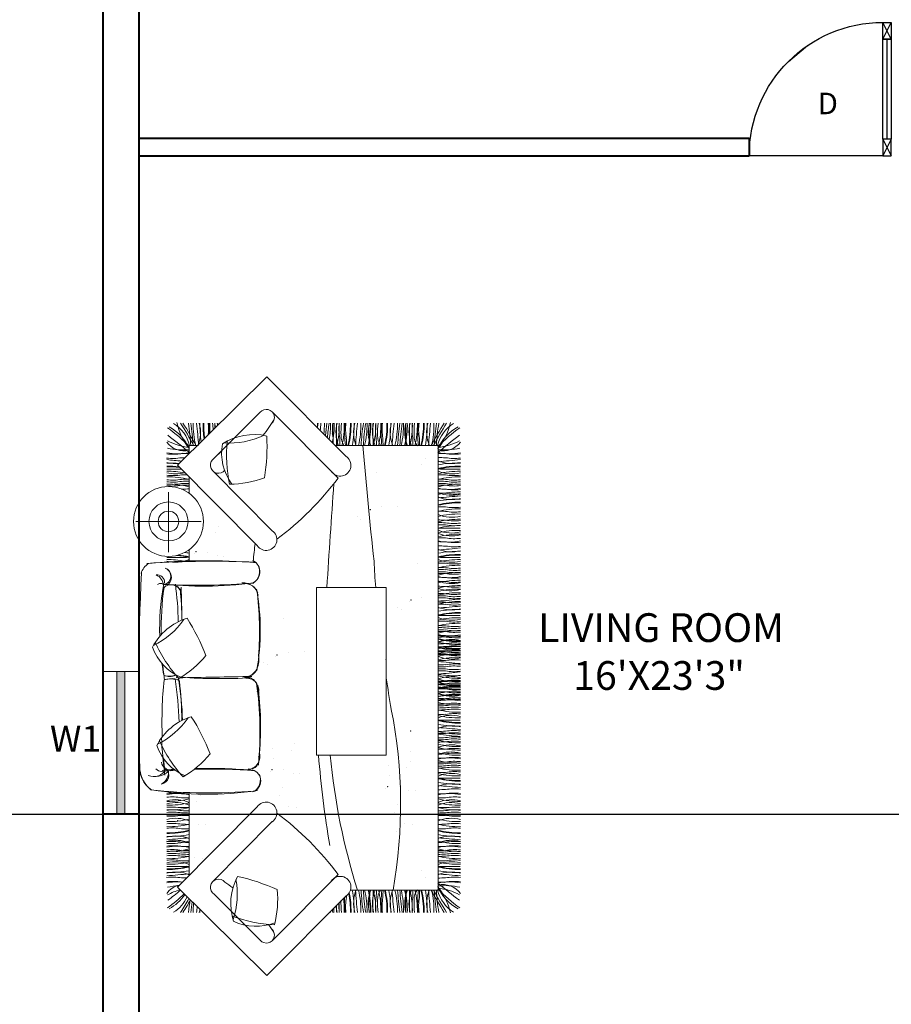
# Model space of a CAD drawing. Units: inches. Extents: x 182 to 1022, y -617 to 111.
# Tile 28 of 33: x 615 to 836, y -337 to -87. Entities that reach past the tile are written whole.
import ezdxf

# ---------------------------------------------------------------- set-up
doc = ezdxf.new("R2010")
doc.units = ezdxf.units.IN
doc.header["$MEASUREMENT"] = 0
for name, color, linetype, lineweight in [('A-ANNO-DIMS', 2, 'Continuous', 18), ('A-ANNO-IDEN', 1, 'Continuous', 18), ('A-AREA-IDEN', 8, 'Continuous', 18), ('A-GLAZ-PATT', 5, 'Continuous', 13), ('door', 2, 'Continuous', 25), ('wall', 1, 'Continuous', 40), ('wind', 5, 'Continuous', 20)]:
    doc.layers.add(name, color=color, linetype=linetype, lineweight=lineweight)
doc.layers.add('furniture', color=50, linetype='Continuous', lineweight=15, transparency=0.8)
doc.styles.get("Standard").update_dxf_attribs({"font": 'arial.ttf'})
doc.dimstyles.get("Standard").update_dxf_attribs({"dimtxt": 0.18, "dimasz": 0.18, "dimexe": 0.18, "dimexo": 0.0625, "dimgap": 0.09, "dimtad": 0, "dimtih": 1, "dimtoh": 1, "dimdec": 1, "dimzin": 0, "dimdsep": 46, "dimlunit": 4, "dimtxsty": 'Standard', "dimcen": 0.09, "dimadec": 0, "dimazin": 0, "dimtfac": 1, "dimtdec": 1, "dimtofl": 0, "dimtmove": 0, "dimatfit": 3, "dimfxl": 1, "dimtolj": 1, "dimtzin": 0, "dimarcsym": 0})

# ---------------------------------------------------------------- blocks, each defined once
blk = doc.blocks.new('A$C2D7661C6')
for p, q in [((0, 700), (50, 800)), ((50, 700), (0, 800)), ((25, 700), (25, 100)), ((50, 100), (0, 0)), ((0, 100), (50, 0))]:
    blk.add_line(p, q)
for points in [[(0, 700), (50, 700), (50, 800), (0, 800)], [(0, 100), (50, 100), (50, 700), (0, 700)], [(0, 100), (50, 100), (50, 0), (0, 0)]]:
    blk.add_lwpolyline(points, close=True)
blk.add_arc((50, 0), 800, 0, 90)
blk = doc.blocks.new('A$C7F556C88')
for p, q in [((615.7, 565.7), (500.3, 661.3)), ((50, 0), (850, 0))]:
    blk.add_line(p, q)
blk.add_blockref('A$C2D7661C6', (0, 0))
blk = doc.blocks.new('LOUNGE-SEATING-GROUP')
for p, q in [((114.94, 73.89), (114.94, 82.17)), ((114.94, 73.89), (107.2, 73.89)), ((114.94, 73.89), (114.94, 65.61)), ((114.94, 73.89), (122.39, 73.89)), ((22.37, 71.64), (0, 48.98)), ((22.37, 71.64), (42.71, 51.42)), ((23.45, 70.43), (23.45, 70.43)), ((23.45, 70.43), (23.45, 70.43)), ((23.45, 70.43), (23.45, 70.43)), ((24.81, 70.1), (24.81, 70.1)), ((24.81, 70.1), (24.81, 70.1)), ((24.81, 70.1), (24.81, 70.1)), ((38.82, 71.99), (38.82, 71.99)), ((41.95, 71.18), (41.95, 71.18)), ((44.62, 71.4), (44.62, 71.4)), ((129.17, 71.64), (108.83, 51.42)), ((129.17, 71.64), (151.54, 48.98)), ((131, 70.1), (131, 70.1)), ((131, 70.1), (131, 70.1)), ((131, 70.1), (131, 70.1)), ((132.36, 70.43), (132.36, 70.43)), ((132.36, 70.43), (132.36, 70.43)), ((132.36, 70.43), (132.36, 70.43)), ((25.37, 68.66), (46.02, 68.66)), ((27.79, 69.24), (27.79, 69.24)), ((27.79, 69.24), (27.79, 69.24)), ((29.83, 67.31), (29.83, 67.31)), ((32.6, 69.72), (32.6, 69.72)), ((34.6, 69.02), (34.6, 69.02)), ((39.15, 68.69), (39.15, 68.69)), ((104.96, 68.66), (107.81, 68.66)), ((106.87, 67.34), (106.87, 67.34)), ((122.07, 68.66), (126.17, 68.66)), ((132.11, 68.66), (134.14, 68.66)), ((134.14, 68.66), (134.14, 66.6)), ((29.68, 65.32), (29.68, 65.32)), ((38.28, 66.24), (38.28, 66.24)), ((44, 66.69), (44, 66.69)), ((45.68, 65.87), (45.68, 65.87)), ((23.81, 62.71), (38.96, 47.66)), ((38.14, 64.53), (38.14, 64.53)), ((107.19, 64.04), (107.19, 64.04)), ((127.73, 62.71), (112.58, 47.66)), ((20.57, 62.3), (8.95, 50.67)), ((20.57, 62.3), (16.28, 58)), ((106.19, 59.88), (106.19, 59.88)), ((106.32, 61.59), (106.32, 61.59)), ((112.04, 62.04), (112.04, 62.04)), ((113.72, 61.22), (113.72, 61.22)), ((130.97, 62.3), (142.59, 50.67)), ((130.97, 62.3), (132.83, 60.43)), ((136.11, 57.16), (142.59, 50.67)), ((12.73, 54.45), (8.95, 50.67)), ((0, 48.98), (20.08, 29.02)), ((25.6, 30.99), (8.82, 47.69)), ((51.77, 48.08), (51.77, 48.08)), ((57.56, 47.49), (57.56, 47.49)), ((78.69, 48.81), (78.69, 48.81)), ((78.69, 48.81), (78.69, 48.81)), ((79.3, 49.74), (79.3, 49.74)), ((79.3, 49.74), (79.3, 49.74)), ((125.94, 30.99), (142.72, 47.69)), ((151.54, 48.98), (131.46, 29.02)), ((40.73, 45.33), (40.73, 45.33)), ((40.73, 45.33), (40.73, 45.33)), ((45.54, 45.81), (45.54, 45.81)), ((47.55, 45.11), (47.55, 45.11)), ((54.89, 47.26), (54.89, 47.26)), ((80.67, 46.7), (80.67, 46.7)), ((42.77, 43.4), (42.77, 43.4)), ((52.09, 44.78), (52.09, 44.78)), ((56.94, 42.77), (56.94, 42.77)), ((81.89, 43.62), (81.89, 43.62)), ((90.41, 44.74), (90.41, 44.74)), ((42.63, 41.41), (42.63, 41.41)), ((51.09, 40.62), (51.09, 40.62)), ((51.22, 42.33), (51.22, 42.33)), ((58.62, 41.96), (58.62, 41.96)), ((81.95, 39.42), (81.95, 39.42)), ((55.77, 18.79), (55.77, 36.47)), ((55.77, 36.47), (98.22, 36.47)), ((98.22, 36.47), (98.22, 18.79)), ((137.17, 32.68), (137.17, 32.68)), ((137.71, 32.64), (137.71, 32.64)), ((134.14, 31.68), (134.14, 5.69)), ((21.66, 5.69), (21.66, 27.82)), ((115.51, 25.24), (115.51, 25.24)), ((115.51, 25.24), (115.51, 25.24)), ((116.12, 26.16), (116.12, 26.16)), ((116.12, 26.16), (116.12, 26.16)), ((18.1, 23.39), (18.1, 23.39)), ((18.64, 23.43), (18.64, 23.43)), ((117.49, 23.12), (117.49, 23.12)), ((137.17, 23.43), (137.17, 23.43)), ((137.71, 23.39), (137.71, 23.39)), ((118.71, 20.04), (118.71, 20.04)), ((127.23, 21.16), (127.23, 21.16)), ((47.45, 18.85), (47.45, 18.85)), ((50.58, 18.04), (50.58, 18.04)), ((53.25, 18.27), (53.25, 18.27)), ((98.22, 18.79), (55.77, 18.79)), ((36.42, 16.11), (36.42, 16.11)), ((36.42, 16.11), (36.42, 16.11)), ((41.23, 16.58), (41.23, 16.58)), ((43.23, 15.88), (43.23, 15.88)), ((47.78, 15.55), (47.78, 15.55)), ((93.22, 15.87), (93.22, 15.87)), ((93.22, 15.87), (93.22, 15.87)), ((118.77, 15.84), (118.77, 15.84)), ((18.1, 14.15), (18.1, 14.15)), ((18.64, 14.19), (18.64, 14.19)), ((38.46, 14.18), (38.46, 14.18)), ((46.91, 13.1), (46.91, 13.1)), ((52.63, 13.55), (52.63, 13.55)), ((54.31, 12.74), (54.31, 12.74)), ((56.63, 12.7), (56.63, 12.7)), ((92.6, 14.94), (92.6, 14.94)), ((92.6, 14.94), (92.6, 14.94)), ((94.58, 12.83), (94.58, 12.83)), ((137.17, 14.19), (137.17, 14.19)), ((137.71, 14.15), (137.71, 14.15)), ((38.31, 12.19), (38.31, 12.19)), ((46.77, 11.39), (46.77, 11.39)), ((104.33, 10.87), (104.33, 10.87)), ((24.84, 8.76), (24.84, 8.76)), ((26.54, 9.97), (26.54, 9.97)), ((95.8, 9.74), (95.8, 9.74)), ((129.27, 9.97), (129.27, 9.97)), ((130.96, 8.76), (130.96, 8.76)), ((134.14, 5.69), (21.66, 5.69)), ((39.44, 5.69), (134.14, 5.69)), ((95.87, 5.55), (95.87, 5.55)), ((23.45, 3.92), (23.45, 3.92)), ((23.45, 3.92), (23.45, 3.92)), ((23.45, 3.92), (23.45, 3.92)), ((24.81, 4.25), (24.81, 4.25)), ((24.81, 4.25), (24.81, 4.25)), ((24.81, 4.25), (24.81, 4.25)), ((69.92, 3.92), (69.92, 3.92)), ((70.05, 3.92), (70.05, 3.92)), ((73.89, 3.92), (73.89, 3.92)), ((81.92, 3.92), (81.92, 3.92)), ((85.76, 3.92), (85.76, 3.92)), ((85.89, 3.92), (85.89, 3.92)), ((131, 4.25), (131, 4.25)), ((131, 4.25), (131, 4.25)), ((131, 4.25), (131, 4.25)), ((132.36, 3.92), (132.36, 3.92)), ((132.36, 3.92), (132.36, 3.92)), ((132.36, 3.92), (132.36, 3.92))]:
    blk.add_line(p, q)
for radius in [8.84, 4.94, 2.61]:
    blk.add_circle((114.94, 73.89), radius)
for centre, radius, start, end in [((52.76, 74.33), 6.91, 83.8792, 147.1093), ((53.34, 72.78), 8.45, 98.6549, 138.7104), ((71.79, -550.87), 632.32, 87.2697, 91.7875), ((100.54, 76.54), 4.47, 31.8817, 73.9672), ((133.78, 64.16), 87.87, 170.8079, 188.3514), ((189.05, 63.59), 142.82, 174.0627, 184.6253), ((53.65, 77.61), 3.29, 154.8715, 246.7247), ((55.6, 77.33), 5.2, 161.2473, 221.1348), ((87.47, 65.64), 13.03, 109.4501, 156.7699), ((76.48, 64.92), 14.61, 17.0126, 62.9429), ((101.32, 86.34), 19.77, 205.9005, 235.6513), ((-54.46, 64.25), 159.48, 355.4325, 5.431), ((-129.18, 62.85), 234.07, 357.3143, 3.933), ((51.47, 77.28), 3.39, 207.8433, 279.8684), ((50.67, 76.05), 2.22, 189.2916, 317.6289), ((73.49, 44.66), 34.51, 114.0815, 132.2768), ((62.54, 64.57), 13.03, 109.4501, 156.7699), ((63.55, -12.93), 88.65, 92.2017, 98.3067), ((54.24, 75.33), 2.63, 137.7203, 204.4461), ((64.36, -31.32), 106.86, 95.0871, 96.7491), ((-77.45, 64.06), 129.9, 3.7101, 5.0653), ((54.5, 73.24), 2.5, 100.6216, 199.193), ((51.55, 63.85), 14.61, 17.0126, 62.9429), ((76.39, 85.27), 19.77, 205.9005, 235.6513), ((64.36, -31.32), 106.86, 84.3639, 92.1219), ((67.78, 73.23), 7.3, 344.0479, 14.2061), ((69.17, 73.11), 6, 351.5362, 18.3493), ((87.05, -6.17), 81.95, 95.7795, 98.522), ((98.42, 45.73), 34.51, 114.0815, 132.2768), ((78.62, 73.56), 2.96, 149.8319, 209.468), ((80.09, 73.77), 4.35, 163.3108, 202.6164), ((87.64, 12.43), 63.7, 97.803, 100.4557), ((87.64, 12.43), 63.7, 79.9466, 91.5903), ((87.05, -6.17), 81.95, 82.1551, 90.5585), ((96.33, 73.24), 2.6, 276.1174, 43.1189), ((189.77, 65.05), 91.22, 172.9836, 187.989), ((98.67, 78.16), 2.97, 271.184, 337.8216), ((97.61, 75.78), 1.68, 314.3938, 33.5856), ((303.26, 66.39), 204.45, 177.5073, 183.9592), ((101.1, 75.54), 2.22, 194.7814, 337.5922), ((99.47, 76.82), 1.96, 268.0108, 6.5585), ((23.91, 77.56), 9.3, 212.2712, 244.6274), ((26.62, 78.75), 10.9, 207.3033, 235.7016), ((48.18, 96.13), 38.02, 215.3153, 223.6457), ((157.47, 180.45), 174.58, 217.5441, 218.8901), ((9.21, 67.69), 12.92, 14.6792, 29.865), ((17.54, 69.88), 5.5, 12.9777, 54.0943), ((7.21, 70.59), 15.55, 2.5322, 13.2785), ((9.4, 71.55), 14.33, 355.1756, 11.2455), ((11.06, 72.81), 12.79, 349.9349, 6.8829), ((12.13, 72.82), 12.79, 349.9349, 6.8829), ((-225.09, 48.88), 251.6, 4.5146, 5.8017), ((17.36, 72.06), 8.84, 337.3098, 14.8613), ((54.69, 73.85), 28.62, 179.0195, 190.4039), ((48.4, 73.82), 21.55, 178.6331, 193.8573), ((48.56, 73.82), 21.55, 178.6331, 193.8573), ((-156.89, 73.02), 184.52, 358.628, 0.3934), ((19.99, 72.06), 8.84, 337.3098, 14.8613), ((49.71, 73.82), 21.55, 178.6331, 193.8573), ((16.48, 72.8), 12.79, 349.9349, 6.8829), ((51.14, 73.82), 21.55, 178.6331, 193.8573), ((17.61, 72.81), 12.79, 349.9349, 6.8829), ((18.12, 72.81), 12.79, 349.9349, 6.8829), ((18.68, 72.81), 12.79, 349.9349, 6.8829), ((52.99, 73.83), 21.55, 178.6331, 193.8573), ((19.1, 72.81), 12.79, 349.9349, 6.8829), ((18.41, 71.55), 14.33, 348.4112, 11.2455), ((20.08, 72.81), 12.79, 349.9349, 6.8829), ((54.95, 73.83), 21.55, 178.6331, 193.8573), ((25.41, 72.08), 8.84, 337.3098, 14.8613), ((21.15, 72.82), 12.79, 349.9349, 6.8829), ((-215.95, 48.88), 251.6, 4.5146, 5.8017), ((26.5, 72.06), 8.84, 337.3098, 14.8613), ((63.83, 73.85), 28.62, 179.0195, 190.4039), ((57.54, 73.82), 21.55, 178.6331, 193.8573), ((57.7, 73.82), 21.55, 178.6331, 193.8573), ((24.58, 72.8), 12.79, 349.9349, 6.8829), ((59.24, 73.82), 21.55, 178.6331, 193.8573), ((25.71, 72.81), 12.79, 349.9349, 6.8829), ((60.52, 73.83), 21.55, 178.6331, 193.8573), ((30.98, 72.08), 8.84, 337.3098, 14.8613), ((61.86, 73.83), 21.55, 178.6331, 193.8573), ((27.93, 72.8), 12.79, 349.9349, 6.8829), ((28.59, 72.81), 12.79, 349.9349, 6.8829), ((29.15, 72.81), 12.79, 349.9349, 6.8829), ((63.46, 73.83), 21.55, 178.6331, 193.8573), ((-141.93, 73.02), 184.52, 358.628, 0.3934), ((34.95, 72.06), 8.84, 337.3098, 14.8613), ((64.67, 73.82), 21.55, 178.6331, 193.8573), ((35.69, 72.06), 8.84, 337.3098, 14.8613), ((65.64, 73.81), 21.55, 178.6331, 193.8573), ((32.43, 72.81), 12.79, 349.9349, 6.8829), ((31.75, 71.55), 14.33, 348.4112, 11.2455), ((33.42, 72.81), 12.79, 349.9349, 6.8829), ((54.09, 73.1), 2.24, 147.7366, 202.2387), ((-105.6, 63.5), 157.88, 3.1908, 3.7892), ((96.83, 72.88), 2.06, 257.6226, 350.3094), ((100.85, 75.64), 2.49, 222.3134, 337.6102), ((113.46, 72.06), 8.84, 165.1387, 202.6902), ((83.74, 73.82), 21.55, 349.3731, 1.3669), ((290.34, 73.02), 184.52, 179.6066, 181.372), ((102.82, 73.83), 21.55, 346.1427, 1.3669), ((136.71, 72.81), 12.79, 173.1171, 190.0651), ((137.13, 72.81), 12.79, 173.1171, 190.0651), ((137.69, 72.81), 12.79, 173.1171, 190.0651), ((138.2, 72.81), 12.79, 173.1171, 190.0651), ((104.67, 73.82), 21.55, 346.1427, 1.3669), ((139.33, 72.8), 12.79, 173.1171, 190.0651), ((135.82, 72.06), 8.84, 165.1387, 194.8341), ((106.1, 73.82), 21.55, 349.2534, 1.3669), ((312.7, 73.02), 184.52, 179.6066, 180.7304), ((107.25, 73.82), 21.55, 352.7707, 1.3669), ((107.41, 73.82), 21.55, 353.2584, 1.3669), ((138.45, 72.06), 8.84, 165.1387, 186.0041), ((101.12, 73.85), 28.62, 354.6488, 0.9805), ((380.9, 48.88), 251.6, 174.1983, 175.0575), ((143.68, 72.82), 12.79, 173.1171, 190.0651), ((144.74, 72.81), 12.79, 173.1171, 190.0651), ((146.41, 71.55), 14.33, 168.7545, 191.5888), ((-1.66, 180.45), 174.58, 320.1568, 322.4559), ((138.27, 69.88), 5.5, 125.9057, 192.8054), ((148.6, 70.59), 15.55, 166.7215, 187.1491), ((129.19, 78.75), 10.9, 292.1181, 332.6967), ((146.6, 67.69), 12.92, 150.135, 175.7243), ((107.63, 96.13), 38.02, 313.716, 324.6847), ((131.9, 77.56), 9.3, 283.9935, 327.7288), ((50.71, 123.35), 63.44, 236.8219, 240.1356), ((50.72, 123.93), 63.44, 236.8219, 240.5026), ((167.37, 66.07), 142.71, 178.1891, 178.6709), ((171.72, 66.06), 142.71, 178.1891, 178.9775), ((172.85, 66.06), 142.71, 178.1891, 178.9775), ((173.36, 66.06), 142.71, 178.1891, 178.9775), ((173.92, 66.06), 142.71, 178.1891, 178.9775), ((174.34, 66.06), 142.71, 178.1891, 178.9775), ((175.32, 66.07), 142.71, 178.1891, 178.9775), ((176.39, 66.07), 142.71, 178.1891, 178.9775), ((179.82, 66.06), 142.71, 178.1891, 178.9775), ((180.95, 66.06), 142.71, 178.1891, 178.9775), ((183.17, 66.05), 142.71, 178.1891, 178.9775), ((183.83, 66.06), 142.71, 178.1891, 178.9775), ((184.39, 66.06), 142.71, 178.1891, 178.9775), ((187.67, 66.06), 142.71, 178.1891, 178.9775), ((188.66, 66.07), 142.71, 178.1891, 178.9775), ((72.34, 83.09), 25.56, 210.3068, 230.5663), ((62.88, 144.51), 73.3, 271.0061, 279.6001), ((63.69, 168.95), 98.42, 270.4949, 276.3291), ((62.39, 148.59), 78.28, 271.6458, 279.5268), ((83.93, 41.27), 31.31, 105.9625, 107.4638), ((90.92, 223.12), 152.58, 263.8872, 264.1215), ((211.78, 60.83), 136.62, 175.8425, 183.2873), ((97.26, 84.16), 25.56, 210.3068, 230.5663), ((76.97, 72.85), 1.85, 209.1313, 222.0141), ((-1557724.04, -27714.17), 1558047.19, 1.02115817, 1.0218453), ((211.78, 60.83), 136.62, 175.3655, 175.4784), ((87.42, 161.02), 89.64, 262.7245, 262.7726), ((87.42, 161.02), 89.64, 271.3731, 277.4472), ((90.92, 223.12), 152.58, 269.6386, 272.7653), ((88.38, 193.19), 122.69, 270.7456, 274.456), ((84.89, 73.82), 21.55, 346.1427, 354.5854), ((85.05, 73.82), 21.55, 346.1427, 353.4467), ((78.77, 73.85), 28.62, 349.5961, 351.862), ((-19.51, 66.07), 142.71, 1.0225, 1.8109), ((-18.53, 66.06), 142.71, 1.0225, 1.8109), ((-18.11, 66.06), 142.71, 1.0225, 1.8109), ((-17.55, 66.06), 142.71, 1.0225, 1.8109), ((-17.04, 66.06), 142.71, 1.0225, 1.8109), ((-15.91, 66.06), 142.71, 1.2964, 1.8109), ((-11.56, 66.07), 142.71, 1.4616, 1.8109), ((-10.5, 66.07), 142.71, 1.0225, 1.8109), ((143.71, 55.46), 16.76, 102.9523, 128.0769), ((105.09, 123.93), 63.44, 297.2669, 303.1781), ((105.1, 123.35), 63.44, 297.2669, 303.1781), ((16.49, 46.09), 21.55, 85.0538, 91.3669), ((25.23, 129.18), 61.61, 261.3771, 263.9203), ((25.24, 129.76), 61.61, 261.3771, 264.3888), ((-105.6, 63.5), 157.88, 355.8027, 1.3803), ((36.21, 114.28), 54.68, 291.3371, 302.4176), ((61.14, 115.35), 54.68, 291.3371, 302.4176), ((-20.58, 66.07), 142.71, 1.0225, 1.0606), ((130.4, 72.08), 8.84, 201.652, 202.6902), ((139.32, 46.09), 21.55, 88.6331, 103.8573), ((130.57, 129.76), 61.61, 273.3644, 278.6229), ((130.58, 129.18), 61.61, 273.3644, 278.6229), ((16.47, 37.31), 28.62, 89.4753, 90.9805), ((18.26, 74.63), 8.84, 255.1387, 260.0752), ((41.44, 317.08), 251.6, 264.1983, 264.5236), ((-77.45, 64.06), 129.9, 354.7422, 1.3335), ((137.55, 74.63), 8.84, 247.3098, 284.8613), ((114.37, 317.08), 251.6, 274.5146, 275.8017), ((139.34, 37.31), 28.62, 89.0195, 98.4847), ((139.31, 43.59), 21.55, 88.6331, 99.2236), ((139.31, 43.43), 21.55, 88.6331, 98.8561), ((22.35, 61.25), 2.06, 307.6748, 149.5181), ((129.19, 61.25), 2.06, 30.4819, 232.3252), ((138.29, 76.55), 12.79, 263.6069, 276.8829), ((137.54, 92.63), 29.12, 269.2987, 274.5064), ((139.31, 41.89), 21.55, 88.6331, 95.2422), ((137.59, 82.54), 19.94, 271.4332, 276.4413), ((132.21, 47.42), 13.03, 79.4501, 126.7699), ((122.34, 52.29), 14.61, 347.0126, 32.9429), ((154.56, 58.42), 19.77, 175.9005, 205.6513), ((139.32, 40.62), 21.55, 88.6331, 92.1135), ((138.3, 74.87), 12.79, 271.3666, 276.8829), ((137.57, 70.15), 8.84, 280.6792, 284.8613), ((138.51, 245.95), 184.52, 270.2284, 270.3934), ((25.49, 51.8), 13.03, 154.4501, 201.7699), ((47.31, 45.46), 34.51, 159.0815, 177.2768), ((18.23, 43.53), 14.61, 62.0126, 107.9429), ((20.65, 76.24), 19.77, 250.9005, 280.6513), ((-9.78, 81.21), 39.77, 323.5454, 327.1144), ((131.74, 24.7), 34.51, 84.0815, 102.2768), ((149.95, 58.56), 25.56, 180.3068, 200.5663), ((-28.28, 68.33), 54.68, 336.3371, 347.4176), ((79.82, 55.6), 4.61, 186.5867, 283.4511), ((95.58, 54.98), 3.83, 280.9756, 4.9747), ((49.28, 53.47), 2.92, 197.7157, 342.8428), ((55.47, 54.17), 3.4, 177.6579, 284.0974), ((54.61, 53.32), 2.35, 170.2617, 291.0115), ((72.28, 54.04), 2.98, 252.9316, 5.1092), ((72.65, 54.26), 2.95, 253.4437, 1.8228), ((78.96, 54.53), 3.36, 174.9234, 245.6374), ((95.69, 54.63), 3.54, 289.8228, 2.4985), ((102.23, 53.89), 3.13, 194.6379, 334.3095), ((102.23, 54.19), 3.33, 213.041, 316.0653), ((219.7, 1090.61), 1044.47, 263.68924, 263.93736), ((10.26, 49.12), 2.03, 130.1092, 319.8908), ((41.21, 49.16), 2.71, 213.6335, 56.3665), ((49.54, 54.15), 3.52, 216.0678, 292.6723), ((61.57, 143.11), 92.36, 264.8245, 277.7148), ((63.01, 128.8), 78.22, 265.0781, 277.695), ((87.31, 108.92), 58.26, 260.0543, 280.4167), ((87.4, 128.63), 77.78, 265.2072, 277.551), ((110.32, 49.16), 2.71, 123.6335, 326.3665), ((161.32, 81.21), 39.77, 231.8457, 238.9133), ((141.28, 49.12), 2.03, 220.1092, 49.8908), ((-9.78, 81.21), 39.77, 301.0867, 304.727), ((134.26, 103.64), 54.68, 261.3371, 272.4176), ((19.32, 71.82), 25.56, 255.3068, 275.5663), ((-19.25, 91.37), 75.22, 306.6049, 323.3387), ((170.79, 91.37), 75.22, 216.6613, 233.3951), ((76.48, -220.38), 257.15, 94.6196, 99.7513), ((114.37, -215), 251.6, 84.1983, 84.6171), ((139.34, 64.77), 28.62, 268.619, 270.9805), ((137.55, 27.45), 8.84, 75.1387, 82.5478), ((16.51, 54.45), 21.55, 268.6331, 269.1046), ((18.25, 23.77), 8.84, 100.6592, 104.8613), ((17.52, 19.64), 12.79, 93.8173, 96.8829), ((22.4, 30.44), 2.72, 211.4693, 56.9076), ((71.51, -132.24), 165.96, 95.4421, 107.4799), ((-225.39, -5012.46), 5056.64, 86.03178, 86.33069), ((129.14, 30.44), 2.72, 123.0924, 328.5307), ((139.32, 53.56), 21.55, 258.2362, 271.3669), ((139.3, 54.45), 21.55, 260.3159, 271.3669), ((138.29, 19.64), 12.79, 83.1171, 100.0651), ((130.57, -27.68), 61.61, 81.3771, 84.7986), ((130.58, -27.11), 61.61, 81.3771, 84.3194), ((139.32, 55.99), 21.55, 263.9229, 271.3669), ((16.49, 53.56), 21.55, 268.6331, 271.5238), ((18.24, 22.68), 8.84, 94.2757, 104.8613), ((16.49, 52.22), 21.55, 268.6331, 274.9238), ((17.51, 17.97), 12.79, 86.2453, 96.8829), ((18.22, 10.3), 19.94, 87.4435, 96.4413), ((17.3, -153.11), 184.52, 89.8849, 90.3934), ((138.51, -153.11), 184.52, 89.6066, 91.372), ((131.55, 173.21), 142.71, 271.0225, 271.8109), ((136.49, 26.38), 3.85, 86.8256, 128.3436), ((139.31, 50.95), 21.55, 256.1427, 271.3669), ((137.57, 22.68), 8.84, 75.1387, 112.6902), ((139.32, 52.22), 21.55, 256.1427, 271.3669), ((131.54, 174.88), 142.71, 271.2535, 271.8109), ((139.31, 53.49), 21.55, 258.0993, 271.3669), ((138.3, 17.97), 12.79, 83.1171, 100.0651), ((137.59, 10.3), 19.94, 83.5587, 92.5565), ((16.5, 50.95), 21.55, 268.6331, 277.9798), ((18.27, 0.21), 29.12, 86.9677, 94.5064), ((17.52, 16.29), 12.79, 79.9349, 96.8829), ((16.5, 49.41), 21.55, 268.6331, 281.3519), ((16.5, 49.25), 21.55, 268.6331, 281.8302), ((24.26, 171.53), 142.71, 268.1891, 268.3576), ((131.55, 171.53), 142.71, 271.0225, 271.8109), ((139.31, 49.25), 21.55, 256.1427, 271.3669), ((139.31, 49.41), 21.55, 256.1427, 271.3669), ((137.54, 0.21), 29.12, 85.4936, 96.6298), ((138.29, 16.29), 12.79, 83.1171, 100.0651), ((16.47, 55.53), 28.62, 269.0195, 280.4039), ((16.49, 46.75), 21.55, 268.6331, 283.8573), ((18.26, 18.21), 8.84, 67.3098, 104.8613), ((25.23, -36.35), 61.61, 93.3644, 98.6229), ((41.44, -224.24), 251.6, 94.5146, 95.8017), ((137.55, 18.21), 8.84, 75.1387, 112.6902), ((139.32, 46.75), 21.55, 256.1427, 271.3669), ((139.34, 55.53), 28.62, 259.5961, 270.9805), ((114.37, -224.24), 251.6, 84.1983, 85.4854), ((130.58, -36.35), 61.61, 81.3771, 86.6356), ((16.49, 44.31), 21.55, 268.6331, 283.8573), ((16.51, 45.2), 21.55, 268.6331, 283.8573), ((18.25, 14.52), 8.84, 67.3098, 104.8613), ((16.5, 44.24), 21.55, 268.6331, 283.8573), ((17.52, 10.39), 12.79, 79.9349, 96.8829), ((25.24, -36.92), 61.61, 93.3644, 98.6229), ((24.27, 165.63), 142.71, 268.1891, 268.9775), ((219.7, -1016.26), 1044.47, 94.69873, 96.31076), ((131.54, 165.63), 142.71, 271.0225, 271.8109), ((139.3, 45.2), 21.55, 256.1427, 271.3669), ((137.55, 14.52), 8.84, 75.1387, 112.6902), ((139.31, 44.24), 21.55, 256.1427, 271.3669), ((139.32, 44.31), 21.55, 256.1427, 271.3669), ((130.57, -36.92), 61.61, 81.3771, 86.6356), ((138.29, 10.39), 12.79, 83.1171, 100.0651), ((18.24, 13.43), 8.84, 67.3098, 104.8613), ((16.49, 42.97), 21.55, 268.6331, 283.8573), ((17.51, 8.72), 12.79, 79.9349, 96.8829), ((18.22, 1.05), 19.94, 87.4435, 96.4413), ((16.5, 41.7), 21.55, 268.6331, 283.8573), ((18.27, -9.04), 29.12, 83.3702, 94.5064), ((17.3, -162.36), 184.52, 88.628, 90.3934), ((19.32, 17.13), 3.85, 51.6564, 93.1744), ((24.26, 163.96), 142.71, 268.1891, 268.9775), ((115.91, -204.23), 226.38, 92.7877, 94.4807), ((138.51, -162.36), 184.52, 89.6066, 91.372), ((131.55, 163.96), 142.71, 271.0225, 271.8109), ((136.49, 17.13), 3.85, 86.8256, 128.3436), ((139.31, 41.7), 21.55, 256.1427, 271.3669), ((137.57, 13.43), 8.84, 75.1387, 112.6902), ((139.32, 42.97), 21.55, 256.1427, 271.3669), ((137.54, -9.04), 29.12, 85.4936, 96.6298), ((138.3, 8.72), 12.79, 83.1171, 100.0651), ((137.59, 1.05), 19.94, 83.5587, 92.5565), ((17.52, 7.04), 12.79, 79.9349, 96.8829), ((16.47, 46.28), 28.62, 269.0195, 280.4039), ((16.5, 40.16), 21.55, 268.6331, 283.8573), ((16.5, 40), 21.55, 268.6331, 283.8573), ((18.26, 8.96), 8.84, 67.3098, 104.8613), ((24.26, 162.28), 142.71, 268.1891, 268.9775), ((43.3, 138.88), 123.73, 259.9275, 281.2246), ((109.32, -219.2), 240.39, 98.119, 100.0442), ((131.55, 162.28), 142.71, 271.0225, 271.8109), ((139.31, 40), 21.55, 256.1427, 271.3669), ((137.55, 8.96), 8.84, 75.1387, 112.6902), ((139.31, 40.16), 21.55, 256.1427, 271.3669), ((139.34, 46.28), 28.62, 259.5961, 270.9805), ((138.29, 7.04), 12.79, 83.1171, 100.0651), ((16.49, 37.5), 21.55, 268.6331, 283.8573), ((25.23, -45.6), 61.61, 93.3644, 98.6229), ((16.51, 35.96), 21.55, 268.6331, 283.8573), ((41.44, -233.49), 251.6, 94.5146, 95.8017), ((25.24, -46.17), 61.61, 93.3644, 98.6229), ((139.3, 35.96), 21.55, 256.1427, 271.3669), ((139.32, 37.5), 21.55, 256.1427, 271.3669), ((114.37, -233.49), 251.6, 84.1983, 85.4854), ((130.57, -46.17), 61.61, 81.3771, 86.6356), ((130.58, -45.6), 61.61, 81.3771, 86.6356), ((16.49, 35.07), 21.55, 268.6331, 283.8573), ((18.24, 4.2), 8.84, 67.3098, 104.8613), ((16.49, 33.73), 21.55, 268.6331, 283.8573), ((18.25, 5.28), 8.84, 67.3098, 104.8613), ((16.5, 35), 21.55, 268.6331, 283.8573), ((17.52, 1.15), 12.79, 79.9349, 96.8829), ((17.3, -171.6), 184.52, 88.628, 90.3934), ((24.27, 156.39), 142.71, 268.1891, 268.9775), ((131.54, 156.39), 142.71, 271.0225, 271.8109), ((138.51, -171.6), 184.52, 89.6066, 91.372), ((137.55, 5.28), 8.84, 75.1387, 112.6902), ((139.31, 35), 21.55, 256.1427, 271.3669), ((139.32, 35.07), 21.55, 256.1427, 271.3669), ((137.57, 4.2), 8.84, 75.1387, 112.6902), ((139.32, 33.73), 21.55, 256.1427, 271.3669), ((138.29, 1.15), 12.79, 83.1171, 100.0651), ((17.51, -0.52), 12.79, 79.9349, 96.8829), ((18.22, -8.19), 19.94, 87.4435, 96.4413), ((16.5, 32.46), 21.55, 268.6331, 283.8573), ((18.27, -18.28), 29.12, 83.3702, 94.5064), ((17.52, -2.2), 12.79, 79.9349, 96.8829), ((16.5, 30.92), 21.55, 268.6331, 283.8573), ((19.32, 7.89), 3.85, 51.6564, 93.1744), ((24.26, 154.72), 142.71, 268.1891, 268.9775), ((24.26, 153.04), 142.71, 268.1891, 268.9775), ((131.55, 153.04), 142.71, 271.0225, 271.8109), ((131.55, 154.72), 142.71, 271.0225, 271.8109), ((136.49, 7.89), 3.85, 86.8256, 128.3436), ((139.31, 32.46), 21.55, 256.1427, 271.3669), ((139.31, 30.92), 21.55, 256.1427, 271.3669), ((137.54, -18.28), 29.12, 85.4936, 96.6298), ((138.3, -0.52), 12.79, 83.1171, 100.0651), ((138.29, -2.2), 12.79, 83.1171, 100.0651), ((137.59, -8.19), 19.94, 83.5587, 92.5565), ((16.47, 37.04), 28.62, 269.0195, 280.4039), ((16.5, 30.76), 21.55, 268.6331, 283.8573), ((18.26, -0.28), 8.84, 67.3098, 104.8613), ((41.44, -242.73), 251.6, 94.5146, 95.8017), ((139.31, 30.76), 21.55, 256.1427, 271.3669), ((137.55, -0.28), 8.84, 75.1387, 112.6902), ((139.34, 37.04), 28.62, 259.5961, 270.9805), ((114.37, -242.73), 251.6, 84.1983, 85.4854), ((12.09, 18.89), 16.76, 282.9523, 308.0769), ((16.49, 28.26), 21.55, 268.6331, 283.8573), ((50.71, -49), 63.44, 117.2669, 123.1781), ((25.23, -54.84), 61.61, 93.3644, 98.6229), ((50.72, -49.58), 63.44, 117.2669, 123.1781), ((25.24, -55.41), 61.61, 93.3644, 98.6229), ((23.91, -3.21), 9.3, 103.9935, 147.7288), ((26.62, -4.4), 10.9, 112.1181, 152.6967), ((48.18, -21.78), 38.02, 133.716, 144.6847), ((157.47, -106.1), 174.58, 140.1568, 142.4559), ((9.21, 6.66), 12.92, 330.135, 355.7243), ((17.54, 4.47), 5.5, 305.9057, 12.8054), ((7.21, 3.76), 15.55, 346.7215, 7.1491), ((9.4, 2.8), 14.33, 348.7545, 11.5888), ((166.3, 8.28), 142.71, 181.0225, 181.8109), ((167.37, 8.28), 142.71, 181.0225, 181.8109), ((-225.09, 25.47), 251.6, 354.1983, 355.4854), ((17.36, 2.29), 8.84, 345.1387, 22.6902), ((54.69, 0.5), 28.62, 169.5961, 180.9805), ((48.4, 0.53), 21.55, 166.1427, 181.3669), ((48.56, 0.53), 21.55, 166.1427, 181.3669), ((-156.89, 1.33), 184.52, 359.6066, 1.372), ((19.99, 2.28), 8.84, 345.1387, 22.6902), ((49.71, 0.53), 21.55, 166.1427, 181.3669), ((171.72, 8.29), 142.71, 181.0225, 181.8109), ((51.14, 0.53), 21.55, 166.1427, 181.3669), ((172.85, 8.29), 142.71, 181.0225, 181.8109), ((173.36, 8.29), 142.71, 181.0225, 181.8109), ((173.92, 8.29), 142.71, 181.0225, 181.8109), ((52.99, 0.52), 21.55, 166.1427, 181.3669), ((174.34, 8.28), 142.71, 181.0225, 181.8109), ((18.41, 2.8), 14.33, 348.7545, 11.5888), ((175.32, 8.28), 142.71, 181.0225, 181.8109), ((54.95, 0.52), 21.55, 166.1427, 181.3669), ((25.41, 2.27), 8.84, 345.1387, 22.6902), ((176.39, 8.28), 142.71, 181.0225, 181.8109), ((-215.95, 25.47), 251.6, 354.1983, 355.4854), ((26.5, 2.29), 8.84, 345.1387, 22.6902), ((63.83, 0.5), 28.62, 169.5961, 180.9805), ((57.54, 0.53), 21.55, 166.1427, 181.3669), ((57.7, 0.53), 21.55, 166.1427, 181.3669), ((179.82, 8.29), 142.71, 181.0225, 181.8109), ((59.24, 0.53), 21.55, 166.1427, 181.3669), ((180.95, 8.29), 142.71, 181.0225, 181.8109), ((60.52, 0.52), 21.55, 166.1427, 181.3669), ((30.98, 2.27), 8.84, 345.1387, 22.6902), ((61.86, 0.52), 21.55, 166.1427, 181.3669), ((183.17, 8.3), 142.71, 181.0225, 181.8109), ((183.83, 8.29), 142.71, 181.0225, 181.8109), ((184.39, 8.29), 142.71, 181.0225, 181.8109), ((63.46, 0.52), 21.55, 166.1427, 181.3669), ((-141.93, 1.33), 184.52, 359.6066, 1.372), ((34.95, 2.28), 8.84, 345.1387, 22.6902), ((64.67, 0.53), 21.55, 166.1427, 181.3669), ((35.69, 2.29), 8.84, 345.1387, 22.6902), ((65.64, 0.54), 21.55, 166.1427, 181.3669), ((187.67, 8.28), 142.71, 181.0225, 181.8109), ((31.75, 2.8), 14.33, 348.7545, 11.5888), ((188.66, 8.28), 142.71, 181.0225, 181.8109), ((189.73, 8.28), 142.71, 181.0225, 181.8109), ((-202.73, 25.47), 251.6, 354.1983, 355.4854), ((39.72, 2.29), 8.84, 345.1387, 22.6902), ((77.04, 0.5), 28.62, 169.5961, 180.9805), ((70.76, 0.53), 21.55, 166.1427, 181.3669), ((70.92, 0.53), 21.55, 166.1427, 181.3669), ((-134.53, 1.33), 184.52, 359.6066, 1.372), ((42.35, 2.28), 8.84, 345.1387, 22.6902), ((72.07, 0.53), 21.55, 166.1427, 181.3669), ((194.08, 8.29), 142.71, 181.0225, 181.8109), ((73.5, 0.53), 21.55, 166.1427, 181.3669), ((195.21, 8.29), 142.71, 181.0225, 181.8109), ((195.71, 8.29), 142.71, 181.0225, 181.8109), ((196.28, 8.29), 142.71, 181.0225, 181.8109), ((75.35, 0.52), 21.55, 166.1427, 181.3669), ((196.69, 8.28), 142.71, 181.0225, 181.8109), ((40.77, 2.8), 14.33, 348.7545, 11.5888), ((197.68, 8.28), 142.71, 181.0225, 181.8109), ((77.31, 0.52), 21.55, 166.1427, 181.3669), ((47.77, 2.27), 8.84, 345.1387, 22.6902), ((198.75, 8.28), 142.71, 181.0225, 181.8109), ((78.64, 0.52), 21.55, 166.1427, 181.3669), ((199.96, 8.3), 142.71, 181.0225, 181.8109), ((49.57, 2.29), 8.84, 345.1387, 22.6902), ((79.51, 0.54), 21.55, 166.1427, 181.3669), ((80.46, 0.54), 21.55, 166.1427, 181.3669), ((201.79, 8.3), 142.71, 181.0225, 181.8109), ((202.36, 8.3), 142.71, 181.0225, 181.8109), ((202.87, 8.28), 142.71, 181.0225, 181.8109), ((536.91, -44.16), 478.45, 174.0165, 174.6992), ((82.68, 0.54), 21.55, 166.1427, 181.3669), ((203.92, 8.31), 142.71, 181.0225, 181.8109), ((204.48, 8.3), 142.71, 181.0225, 181.8109), ((-188.03, 25.47), 251.6, 354.1983, 355.4854), ((54.41, 2.29), 8.84, 345.1387, 22.6902), ((91.74, 0.5), 28.62, 169.5961, 180.9805), ((85.45, 0.53), 21.55, 166.1427, 181.3669), ((85.62, 0.53), 21.55, 166.1427, 181.3669), ((-119.83, 1.33), 184.52, 359.6066, 1.372), ((57.05, 2.28), 8.84, 345.1387, 22.6902), ((86.77, 0.53), 21.55, 166.1427, 181.3669), ((208.77, 8.29), 142.71, 181.0225, 181.8109), ((88.19, 0.53), 21.55, 166.1427, 181.3669), ((209.9, 8.29), 142.71, 181.0225, 181.8109), ((210.41, 8.29), 142.71, 181.0225, 181.8109), ((210.97, 8.29), 142.71, 181.0225, 181.8109), ((90.05, 0.52), 21.55, 166.1427, 181.3669), ((211.39, 8.28), 142.71, 181.0225, 181.8109), ((55.47, 2.8), 14.33, 348.7545, 11.5888), ((212.38, 8.28), 142.71, 181.0225, 181.8109), ((48.78, 0.54), 21.55, 358.6331, 13.8573), ((-72.55, 8.3), 142.71, 358.1891, 358.9775), ((49.6, 0.54), 21.55, 358.6331, 13.8573), ((49.72, 0.54), 21.55, 358.6331, 13.8573), ((79.54, 2.29), 8.84, 157.3098, 194.8613), ((79.66, 2.29), 8.84, 157.3098, 194.8613), ((50.47, 0.52), 21.55, 358.6331, 13.8573), ((-70.85, 8.3), 142.71, 358.1891, 358.9775), ((94.05, 0.52), 21.55, 166.1427, 181.3669), ((-70.1, 8.31), 142.71, 358.1891, 358.9775), ((64.51, 2.27), 8.84, 345.1387, 22.6902), ((-403.08, -44.16), 478.45, 5.3008, 5.9835), ((215.49, 8.28), 142.71, 181.0225, 181.8109), ((-69.05, 8.28), 142.71, 358.1891, 358.9775), ((95.15, 0.54), 21.55, 166.1427, 181.3669), ((216.49, 8.3), 142.71, 181.0225, 181.8109), ((217.05, 8.3), 142.71, 181.0225, 181.8109), ((95.91, 0.52), 21.55, 166.1427, 181.3669), ((217.23, 8.3), 142.71, 181.0225, 181.8109), ((66.84, 2.29), 8.84, 345.1387, 22.6902), ((96.78, 0.54), 21.55, 166.1427, 181.3669), ((-66.58, 8.31), 142.71, 358.1891, 358.9775), ((-399.56, -44.16), 478.45, 5.3008, 5.9835), ((-65.53, 8.28), 142.71, 358.1891, 358.9775), ((-65.01, 8.3), 142.71, 358.1891, 358.9775), ((220.82, 8.3), 142.71, 181.0225, 181.8109), ((221.34, 8.28), 142.71, 181.0225, 181.8109), ((555.37, -44.16), 478.45, 174.0165, 174.6992), ((222.39, 8.31), 142.71, 181.0225, 181.8109), ((59.03, 0.54), 21.55, 358.6331, 13.8573), ((88.97, 2.29), 8.84, 157.3098, 194.8613), ((59.9, 0.52), 21.55, 358.6331, 13.8573), ((-61.42, 8.3), 142.71, 358.1891, 358.9775), ((-61.24, 8.3), 142.71, 358.1891, 358.9775), ((60.65, 0.54), 21.55, 358.6331, 13.8573), ((-60.68, 8.3), 142.71, 358.1891, 358.9775), ((224.85, 8.28), 142.71, 181.0225, 181.8109), ((91.3, 2.27), 8.84, 157.3098, 194.8613), ((558.89, -44.16), 478.45, 174.0165, 174.6992), ((61.76, 0.52), 21.55, 358.6331, 13.8573), ((-59.68, 8.28), 142.71, 358.1891, 358.9775), ((225.91, 8.31), 142.71, 181.0225, 181.8109), ((105.34, 0.52), 21.55, 166.1427, 181.3669), ((226.66, 8.3), 142.71, 181.0225, 181.8109), ((76.15, 2.29), 8.84, 345.1387, 22.6902), ((76.27, 2.29), 8.84, 345.1387, 22.6902), ((106.09, 0.54), 21.55, 166.1427, 181.3669), ((106.21, 0.54), 21.55, 166.1427, 181.3669), ((107.03, 0.54), 21.55, 166.1427, 181.3669), ((228.36, 8.3), 142.71, 181.0225, 181.8109), ((100.34, 2.8), 14.33, 168.4112, 191.2455), ((-56.57, 8.28), 142.71, 358.1891, 358.9775), ((65.76, 0.52), 21.55, 358.6331, 13.8573), ((-55.58, 8.28), 142.71, 358.1891, 358.9775), ((-55.17, 8.29), 142.71, 358.1891, 358.9775), ((-54.6, 8.29), 142.71, 358.1891, 358.9775), ((67.62, 0.53), 21.55, 358.6331, 13.8573), ((-54.1, 8.29), 142.71, 358.1891, 358.9775), ((-52.96, 8.29), 142.71, 358.1891, 358.9775), ((98.76, 2.28), 8.84, 157.3098, 194.8613), ((69.04, 0.53), 21.55, 358.6331, 13.8573), ((275.64, 1.33), 184.52, 178.628, 180.3934), ((70.19, 0.53), 21.55, 358.6331, 13.8573), ((70.35, 0.53), 21.55, 358.6331, 13.8573), ((64.07, 0.5), 28.62, 359.0195, 10.4039), ((101.4, 2.29), 8.84, 157.3098, 194.8613), ((343.84, 25.47), 251.6, 184.5146, 185.8017), ((-48.67, 8.3), 142.71, 358.1891, 358.9775), ((73.12, 0.54), 21.55, 358.6331, 13.8573), ((-48.12, 8.31), 142.71, 358.1891, 358.9775), ((-381.1, -44.16), 478.45, 5.3008, 5.9835), ((-47.06, 8.28), 142.71, 358.1891, 358.9775), ((-46.55, 8.3), 142.71, 358.1891, 358.9775), ((75.35, 0.54), 21.55, 358.6331, 13.8573), ((-45.98, 8.3), 142.71, 358.1891, 358.9775), ((76.29, 0.54), 21.55, 358.6331, 13.8573), ((106.23, 2.29), 8.84, 157.3098, 194.8613), ((77.16, 0.52), 21.55, 358.6331, 13.8573), ((-44.15, 8.3), 142.71, 358.1891, 358.9775), ((108.04, 2.27), 8.84, 157.3098, 194.8613), ((78.5, 0.52), 21.55, 358.6331, 13.8573), ((-42.94, 8.28), 142.71, 358.1891, 358.9775), ((115.04, 2.8), 14.33, 168.4112, 191.2455), ((-41.87, 8.28), 142.71, 358.1891, 358.9775), ((80.46, 0.52), 21.55, 358.6331, 13.8573), ((-40.88, 8.28), 142.71, 358.1891, 358.9775), ((-40.47, 8.29), 142.71, 358.1891, 358.9775), ((-39.9, 8.29), 142.71, 358.1891, 358.9775), ((82.31, 0.53), 21.55, 358.6331, 13.8573), ((-39.4, 8.29), 142.71, 358.1891, 358.9775), ((-38.27, 8.29), 142.71, 358.1891, 358.9775), ((113.46, 2.28), 8.84, 157.3098, 194.8613), ((83.74, 0.53), 21.55, 358.6331, 13.8573), ((290.34, 1.33), 184.52, 178.628, 180.3934), ((84.89, 0.53), 21.55, 358.6331, 13.8573), ((85.05, 0.53), 21.55, 358.6331, 13.8573), ((78.77, 0.5), 28.62, 359.0195, 10.4039), ((116.09, 2.29), 8.84, 157.3098, 194.8613), ((358.54, 25.47), 251.6, 184.5146, 185.8017), ((-33.92, 8.28), 142.71, 358.1891, 358.9775), ((124.06, 2.8), 14.33, 168.4112, 191.2455), ((-32.85, 8.28), 142.71, 358.1891, 358.9775), ((-31.87, 8.28), 142.71, 358.1891, 358.9775), ((90.17, 0.54), 21.55, 358.6331, 13.8573), ((120.11, 2.29), 8.84, 157.3098, 194.8613), ((120.86, 2.28), 8.84, 157.3098, 194.8613), ((91.14, 0.53), 21.55, 358.6331, 13.8573), ((297.74, 1.33), 184.52, 178.628, 180.3934), ((92.34, 0.52), 21.55, 358.6331, 13.8573), ((-28.58, 8.29), 142.71, 358.1891, 358.9775), ((-28.02, 8.29), 142.71, 358.1891, 358.9775), ((93.95, 0.52), 21.55, 358.6331, 13.8573), ((-27.36, 8.3), 142.71, 358.1891, 358.9775), ((124.83, 2.27), 8.84, 157.3098, 194.8613), ((95.29, 0.52), 21.55, 358.6331, 13.8573), ((96.57, 0.53), 21.55, 358.6331, 13.8573), ((-25.14, 8.29), 142.71, 358.1891, 358.9775), ((-24.01, 8.29), 142.71, 358.1891, 358.9775), ((98.11, 0.53), 21.55, 358.6331, 13.8573), ((98.27, 0.53), 21.55, 358.6331, 13.8573), ((91.98, 0.5), 28.62, 359.0195, 10.4039), ((129.31, 2.29), 8.84, 157.3098, 194.8613), ((371.75, 25.47), 251.6, 184.5146, 185.8017), ((130.4, 2.27), 8.84, 157.3098, 194.8613), ((100.86, 0.52), 21.55, 358.6331, 13.8573), ((-20.58, 8.28), 142.71, 358.1891, 358.9775), ((137.39, 2.8), 14.33, 168.4112, 191.2455), ((-19.51, 8.28), 142.71, 358.1891, 358.9775), ((102.82, 0.52), 21.55, 358.6331, 13.8573), ((-18.53, 8.28), 142.71, 358.1891, 358.9775), ((-18.11, 8.29), 142.71, 358.1891, 358.9775), ((-17.55, 8.29), 142.71, 358.1891, 358.9775), ((-17.04, 8.29), 142.71, 358.1891, 358.9775), ((104.67, 0.53), 21.55, 358.6331, 13.8573), ((-15.91, 8.29), 142.71, 358.1891, 358.9775), ((135.82, 2.28), 8.84, 157.3098, 194.8613), ((106.1, 0.53), 21.55, 358.6331, 13.8573), ((107.25, 0.53), 21.55, 358.6331, 13.8573), ((312.7, 1.33), 184.52, 178.628, 180.3934), ((107.41, 0.53), 21.55, 358.6331, 13.8573), ((101.12, 0.5), 28.62, 359.0195, 10.4039), ((138.45, 2.29), 8.84, 157.3098, 194.8613), ((380.9, 25.47), 251.6, 184.5146, 185.8017), ((-11.56, 8.28), 142.71, 358.1891, 358.9775), ((146.41, 2.8), 14.33, 168.4112, 191.2455), ((-10.5, 8.28), 142.71, 358.1891, 358.9775), ((-1.66, -106.1), 174.58, 37.5441, 39.8432), ((138.27, 4.47), 5.5, 167.1946, 234.0943), ((148.6, 3.76), 15.55, 172.8509, 193.2785), ((129.19, -4.4), 10.9, 27.3033, 67.8819), ((143.71, 18.89), 16.76, 231.9231, 257.0477), ((146.6, 6.66), 12.92, 184.2757, 209.865), ((107.63, -21.78), 38.02, 35.3153, 46.284), ((105.09, -49.58), 63.44, 56.8219, 62.7331), ((131.9, -3.21), 9.3, 32.2712, 76.0065), ((105.1, -49), 63.44, 56.8219, 62.7331), ((139.32, 28.26), 21.55, 256.1427, 271.3669), ((130.57, -55.41), 61.61, 81.3771, 86.6356), ((130.58, -54.84), 61.61, 81.3771, 86.6356), ((11.06, 1.54), 12.79, 353.1171, 10.0651), ((12.13, 1.53), 12.79, 353.1171, 10.0651), ((16.48, 1.55), 12.79, 353.1171, 10.0651), ((17.61, 1.54), 12.79, 353.1171, 10.0651), ((18.12, 1.54), 12.79, 353.1171, 10.0651), ((18.68, 1.54), 12.79, 353.1171, 10.0651), ((19.1, 1.54), 12.79, 353.1171, 10.0651), ((20.08, 1.54), 12.79, 353.1171, 10.0651), ((21.15, 1.53), 12.79, 353.1171, 10.0651), ((24.58, 1.55), 12.79, 353.1171, 10.0651), ((25.71, 1.54), 12.79, 353.1171, 10.0651), ((27.93, 1.55), 12.79, 353.1171, 10.0651), ((28.59, 1.54), 12.79, 353.1171, 10.0651), ((29.15, 1.54), 12.79, 353.1171, 10.0651), ((32.43, 1.54), 12.79, 353.1171, 10.0651), ((33.42, 1.54), 12.79, 353.1171, 10.0651), ((34.49, 1.53), 12.79, 353.1171, 10.0651), ((38.84, 1.55), 12.79, 353.1171, 10.0651), ((39.97, 1.54), 12.79, 353.1171, 10.0651), ((40.47, 1.54), 12.79, 353.1171, 10.0651), ((41.04, 1.54), 12.79, 353.1171, 10.0651), ((41.45, 1.54), 12.79, 353.1171, 10.0651), ((42.44, 1.54), 12.79, 353.1171, 10.0651), ((43.51, 1.53), 12.79, 353.1171, 10.0651), ((44.72, 1.55), 12.79, 353.1171, 10.0651), ((46.55, 1.55), 12.79, 353.1171, 10.0651), ((47.12, 1.55), 12.79, 353.1171, 10.0651), ((47.63, 1.53), 12.79, 353.1171, 10.0651), ((48.68, 1.56), 12.79, 353.1171, 10.0651), ((49.24, 1.56), 12.79, 353.1171, 10.0651), ((53.53, 1.55), 12.79, 353.1171, 10.0651), ((54.66, 1.54), 12.79, 353.1171, 10.0651), ((55.17, 1.54), 12.79, 353.1171, 10.0651), ((55.73, 1.54), 12.79, 353.1171, 10.0651), ((56.15, 1.54), 12.79, 353.1171, 10.0651), ((57.14, 1.54), 12.79, 353.1171, 10.0651), ((82.69, 1.55), 12.79, 169.9349, 186.8829), ((84.39, 1.55), 12.79, 169.9349, 186.8829), ((85.14, 1.56), 12.79, 169.9349, 186.8829), ((60.25, 1.53), 12.79, 353.1171, 10.0651), ((86.19, 1.53), 12.79, 169.9349, 186.8829), ((61.25, 1.55), 12.79, 353.1171, 10.0651), ((61.81, 1.55), 12.79, 353.1171, 10.0651), ((61.99, 1.55), 12.79, 353.1171, 10.0651), ((88.66, 1.56), 12.79, 169.9349, 186.8829), ((89.71, 1.53), 12.79, 169.9349, 186.8829), ((90.23, 1.55), 12.79, 169.9349, 186.8829), ((65.58, 1.55), 12.79, 353.1171, 10.0651), ((66.1, 1.53), 12.79, 353.1171, 10.0651), ((67.15, 1.56), 12.79, 353.1171, 10.0651), ((93.82, 1.55), 12.79, 169.9349, 186.8829), ((94, 1.55), 12.79, 169.9349, 186.8829), ((94.56, 1.55), 12.79, 169.9349, 186.8829), ((69.61, 1.53), 12.79, 353.1171, 10.0651), ((95.56, 1.53), 12.79, 169.9349, 186.8829), ((70.67, 1.56), 12.79, 353.1171, 10.0651), ((71.42, 1.55), 12.79, 353.1171, 10.0651), ((73.12, 1.55), 12.79, 353.1171, 10.0651), ((98.67, 1.54), 12.79, 169.9349, 186.8829), ((99.66, 1.54), 12.79, 169.9349, 186.8829), ((100.07, 1.54), 12.79, 169.9349, 186.8829), ((100.64, 1.54), 12.79, 169.9349, 186.8829), ((101.14, 1.54), 12.79, 169.9349, 186.8829), ((102.28, 1.55), 12.79, 169.9349, 186.8829), ((106.57, 1.56), 12.79, 169.9349, 186.8829), ((107.12, 1.56), 12.79, 169.9349, 186.8829), ((108.18, 1.53), 12.79, 169.9349, 186.8829), ((108.69, 1.55), 12.79, 169.9349, 186.8829), ((109.26, 1.55), 12.79, 169.9349, 186.8829), ((111.09, 1.55), 12.79, 169.9349, 186.8829), ((112.3, 1.53), 12.79, 169.9349, 186.8829), ((113.37, 1.54), 12.79, 169.9349, 186.8829), ((114.36, 1.54), 12.79, 169.9349, 186.8829), ((114.77, 1.54), 12.79, 169.9349, 186.8829), ((115.34, 1.54), 12.79, 169.9349, 186.8829), ((115.84, 1.54), 12.79, 169.9349, 186.8829), ((116.97, 1.55), 12.79, 169.9349, 186.8829), ((121.32, 1.53), 12.79, 169.9349, 186.8829), ((122.39, 1.54), 12.79, 169.9349, 186.8829), ((123.37, 1.54), 12.79, 169.9349, 186.8829), ((126.66, 1.54), 12.79, 169.9349, 186.8829), ((127.22, 1.54), 12.79, 169.9349, 186.8829), ((127.88, 1.55), 12.79, 169.9349, 186.8829), ((130.1, 1.54), 12.79, 169.9349, 186.8829), ((131.23, 1.55), 12.79, 169.9349, 186.8829), ((134.66, 1.53), 12.79, 169.9349, 186.8829), ((135.73, 1.54), 12.79, 169.9349, 186.8829), ((136.71, 1.54), 12.79, 169.9349, 186.8829), ((137.13, 1.54), 12.79, 169.9349, 186.8829), ((137.69, 1.54), 12.79, 169.9349, 186.8829), ((138.2, 1.54), 12.79, 169.9349, 186.8829), ((139.33, 1.55), 12.79, 169.9349, 186.8829), ((143.68, 1.53), 12.79, 169.9349, 186.8829), ((144.74, 1.54), 12.79, 169.9349, 186.8829)]:
    blk.add_arc(centre, radius, start, end)
for p in [(39.21, 71.6), (107.26, 66.95), (52.16, 47.69), (81.15, 46.43), (117.97, 22.85), (47.84, 18.46), (80.04, 18.85), (61.92, 12.58), (95.07, 12.56)]:
    blk.add_point(p)
blk = doc.blocks.new('*D39')
at = {"layer": 'A-ANNO-DIMS', "color": 0, "lineweight": -2, "transparency": 16777216}
for p, q in [((238.4, -288.54), (1015.28, -288.54)), ((1015.1, -288.72), (1015.1, -346.77)), ((1015.1, -405.19), (1015.1, -347.14)), ((238.43, -405.37), (1015.28, -405.37))]:
    blk.add_line(p, q, dxfattribs=at)
at = {"layer": 'A-ANNO-DIMS', "color": 0, "transparency": 16777216}
for points in [[(1015.07, -288.72), (1015.13, -288.72), (1015.1, -288.54)], [(1015.07, -405.19), (1015.13, -405.19), (1015.1, -405.37)]]:
    blk.add_solid(points, dxfattribs=at)
at = {"layer": 'Defpoints', "color": 0, "transparency": 16777216}
for p in [(238.34, -288.54), (1015.1, -288.54), (238.36, -405.37)]:
    blk.add_point(p, dxfattribs=at)
at = {"layer": 'A-ANNO-DIMS', "color": 0, "transparency": 16777216, "insert": (1015.1, -346.96), "char_height": 0.18, "attachment_point": 5}
blk.add_mtext('\\A1;9\'-9"', dxfattribs=at)

msp = doc.modelspace()

# ---------------------------------------------------------------- hatches: boundary and pattern name
at = {"layer": 'A-GLAZ-PATT'}
h = msp.add_hatch(color=256, dxfattribs=at)
h.dxf.hatch_style = 1
h.paths.add_polyline_path([(692.35, -3.87), (662.35, -3.87), (662.35, -5.87), (692.35, -5.87)])
h.paths.add_polyline_path([(783.03, -3.87), (747.03, -3.87), (747.03, -5.87), (783.03, -5.87)])
h.paths.add_polyline_path([(641.8, -252.37), (639.8, -252.37), (639.8, -288.37), (641.8, -288.37)])
h.paths.add_polyline_path([(968.8, -258.37), (966.8, -258.37), (966.8, -282.37), (968.8, -282.37)])
h.paths.add_polyline_path([(968.8, -132.92), (966.8, -132.92), (966.8, -168.92), (968.8, -168.92)])
h.paths.add_polyline_path([(940.3, -534.87), (904.3, -534.87), (904.3, -536.87), (940.3, -536.87)])

# ---------------------------------------------------------------- linework, layer by layer
at = {"layer": 'wall'}
for p, q in [((636.3, -540.37), (636.3, -0.37)), ((645.3, -9.37), (645.3, -540.37)), ((645.3, -117.37), (799.8, -117.37)), ((799.8, -117.37), (799.8, -121.87)), ((645.3, -121.87), (799.8, -121.87))]:
    msp.add_line(p, q, dxfattribs=at)
at = {"layer": 'wind'}
for p, q in [((636.3, -252.37), (645.3, -252.37)), ((639.8, -252.37), (639.8, -288.37)), ((641.8, -252.37), (641.8, -288.37)), ((636.3, -288.37), (645.3, -288.37))]:
    msp.add_line(p, q, dxfattribs=at)

# ---------------------------------------------------------------- block references
at = {"layer": 'door', "xscale": -0.042214023418219, "yscale": 0.042214023418219, "zscale": 0.042214023418219}
msp.add_blockref('A$C7F556C88', (835.69, -121.87), dxfattribs=at)
at = {"layer": 'furniture', "rotation": 90}
msp.add_blockref('LOUNGE-SEATING-GROUP', (726.73, -329.37), dxfattribs=at)

# ---------------------------------------------------------------- texts
at = {"layer": 'A-ANNO-IDEN'}
for s, height, p in [('D', 5.44, (817.13, -111.34)), ('W1', 6.652, (622.84, -272.73))]:
    msp.add_text(s, height=height, dxfattribs=at).set_placement(p)
at = {"layer": 'A-AREA-IDEN', "insert": (737.5, -237.66), "char_height": 7.2703, "attachment_point": 1}
msp.add_mtext_dynamic_manual_height_columns('    LIVING ROOM\\P        16\'X23\'3"', width=90.7812, gutter_width=1.21, heights=[0], dxfattribs=at)

# ---------------------------------------------------------------- dimensions: what is measured, and where the dimension line sits
at = {"layer": 'A-ANNO-DIMS'}
dim = msp.add_linear_dim(base=(1015.1, -288.54), p1=(238.36, -405.37), p2=(238.34, -288.54), angle=90, dimstyle='Standard', override={"dimdec": 1, "dimlfac": 1, "dimrnd": 0, "dimzin": 1, "dimdsep": 46, "dimlunit": 4, "dimfrac": 2}, dxfattribs=at)
dim.commit()
dim.dimension.update_dxf_attribs({"geometry": '*D39', "text_midpoint": (1015.1, -346.96)})

doc.saveas('drawing.dxf')
